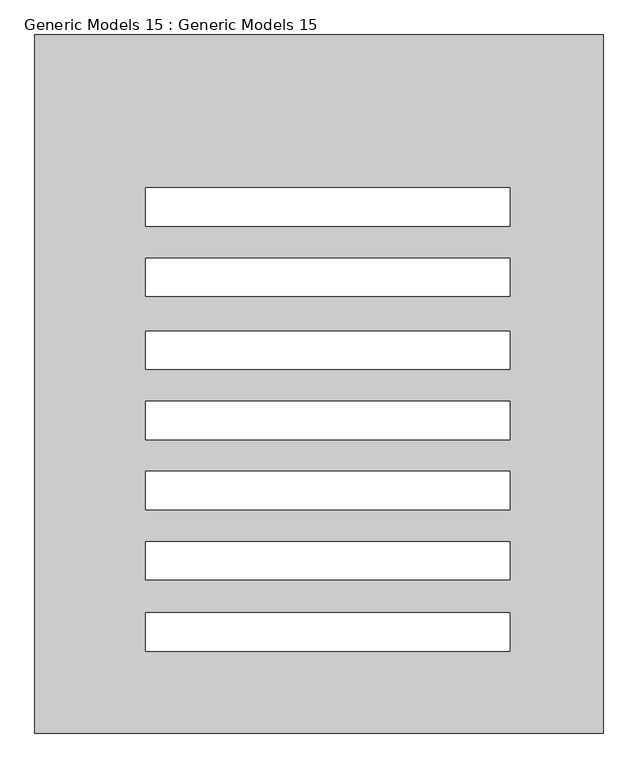
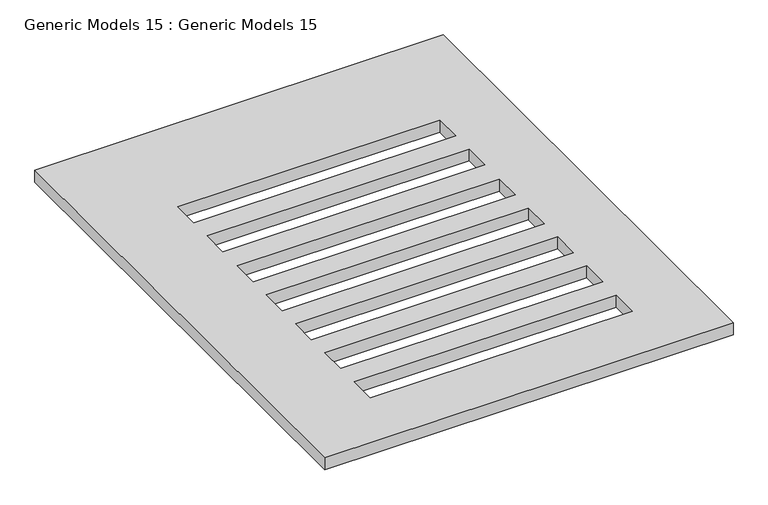
"""IFC4 building model written with IfcOpenShell, lengths in millimetres: proxy geometry, Generic Models 15 : Generic Models 15."""

from ifc_helpers import new_model, si_unit, frame, origin, place, context, project, spatial, polyline, outline, extrude, source, transform, mapped, element, save


def generic_models_15_generic_models_15_5c454abc(model_context):
    return source(origin(), model_context, "Body", "SweptSolid", [
        extrude(outline(polyline([(7481.8271899, -11497.4679047), (7481.8271899, -5431.2794704), (12422.4804136, -5431.2794704), (12422.4804136, -11497.4679047), (7481.8271899, -11497.4679047)]), holes=[polyline([(8444.2128058, -10784.6551138), (11612.466985, -10784.6551138), (11612.466985, -10451.9357332), (8444.2128058, -10451.9357332), (8444.2128058, -10784.6551138)]), polyline([(8444.2128058, -10166.4872853), (11612.466985, -10166.4872853), (11612.466985, -9833.7679047), (8444.2128058, -9833.7679047), (8444.2128058, -10166.4872853)]), polyline([(8444.2128058, -9556.8872853), (11612.466985, -9556.8872853), (11612.466985, -9224.1679047), (8444.2128058, -9224.1679047), (8444.2128058, -9556.8872853)]), polyline([(8444.2128058, -8947.2872853), (11612.466985, -8947.2872853), (11612.466985, -8614.5679047), (8444.2128058, -8614.5679047), (8444.2128058, -8947.2872853)]), polyline([(8444.2128058, -8337.6872853), (11612.466985, -8337.6872853), (11612.466985, -8004.9679047), (8444.2128058, -8004.9679047), (8444.2128058, -8337.6872853)]), polyline([(8444.2128058, -7702.6872853), (11612.466985, -7702.6872853), (11612.466985, -7369.9679047), (8444.2128058, -7369.9679047), (8444.2128058, -7702.6872853)]), polyline([(8444.2128058, -7093.0872853), (11612.466985, -7093.0872853), (11612.466985, -6760.3679047), (8444.2128058, -6760.3679047), (8444.2128058, -7093.0872853)])]), frame((0.0, 0.0, 15240.0), z_axis=(0.0, 0.0, 1.0), x_axis=(1.0, 0.0, 0.0)), (0.0, 0.0, 1.0), 152.4),
    ])


if __name__ == "__main__":
    model = new_model("IFC4")
    model_context = context("Model", 3, world=origin())
    ifc_project = project(units=[si_unit("LENGTHUNIT", "METRE", prefix="MILLI")], contexts=[model_context])
    site = spatial("IfcSite", under=ifc_project)
    building = spatial("IfcBuilding", under=site)
    placement = place(None, origin())
    generic_models_15_generic_models_15_shape = generic_models_15_generic_models_15_5c454abc(model_context)
    element("IfcBuildingElementProxy", 1, Name="Generic Models 15 : Generic Models 15", ObjectType="Generic Models 15 : Generic Models 15", at=placement, inside=building, context=model_context, shape_type="MappedRepresentation", body=[
        mapped(generic_models_15_generic_models_15_shape, transform((0.0, 0.0, 0.0), x_axis=(1.0, 0.0, 0.0), y_axis=(0.0, 1.0, 0.0), z_axis=(0.0, 0.0, 1.0))),
    ])
    save(model, "model.ifc")

# Revit data of these elements
# Element 1 (IfcBuildingElementProxy, "Generic Models 15 : Generic Models 15")
#   Materials on its faces: "TEAK BROWN COLOUR"
# Materials
#   "TEAK BROWN COLOUR": class "Generic", colour RGB 120 120 120, transparency 0, Cost = 0
